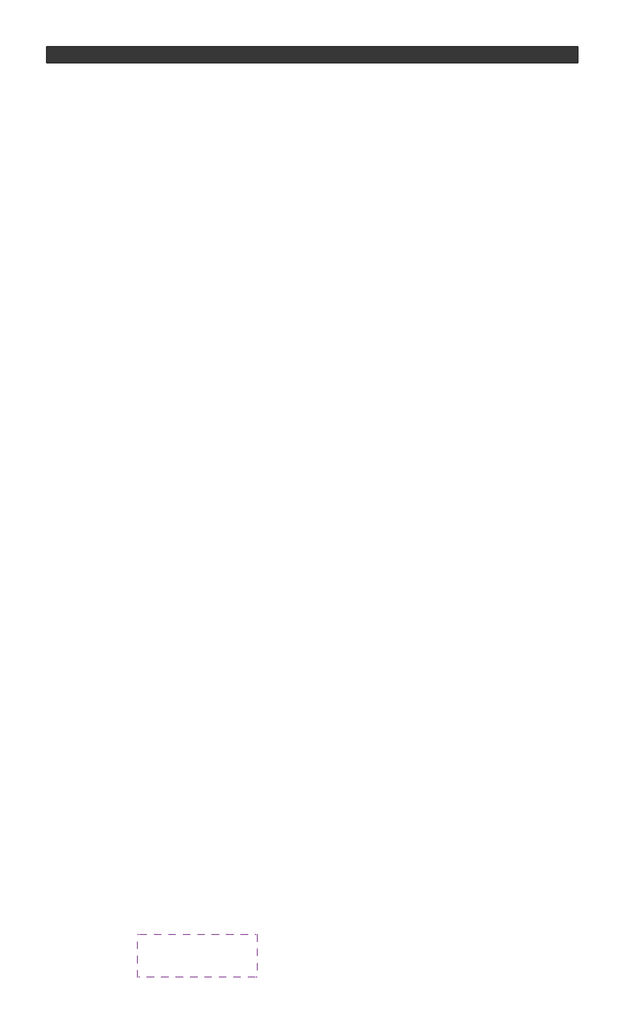
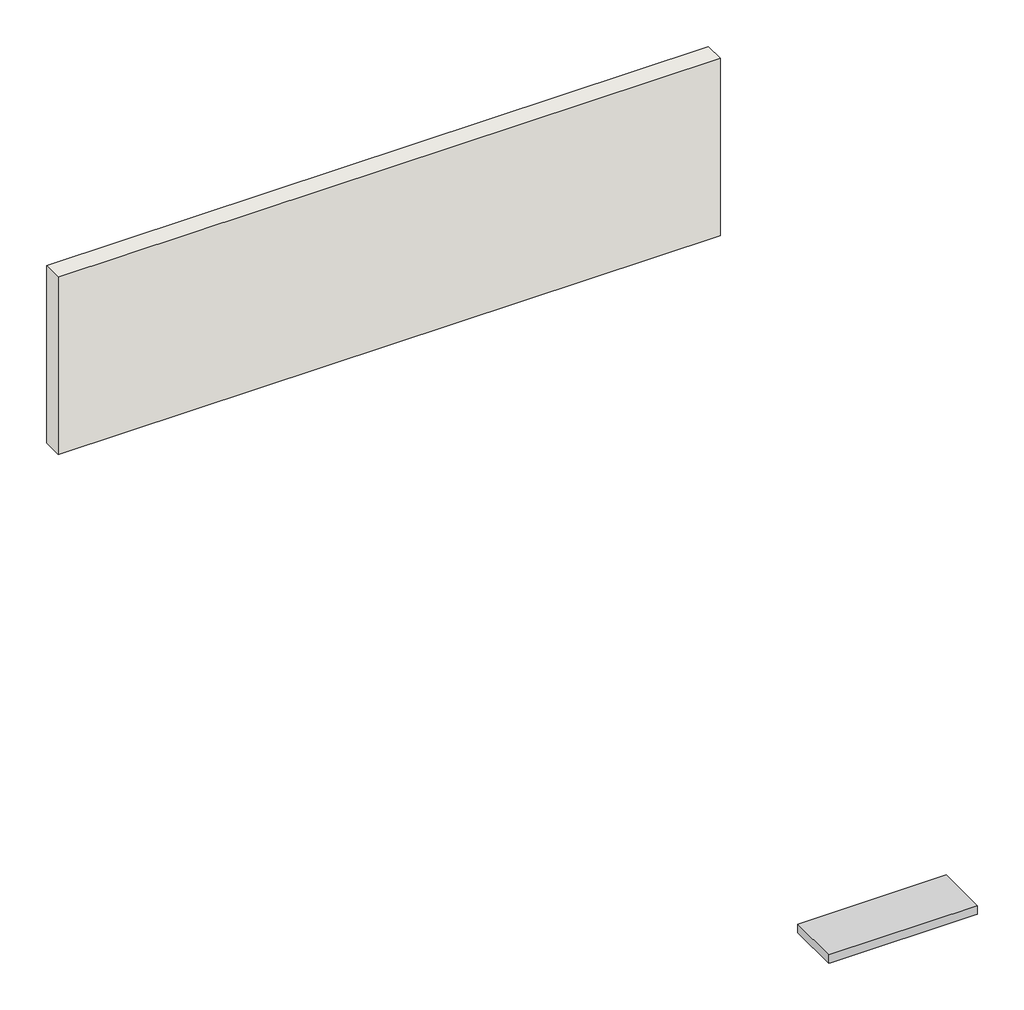
# One storey: 1 proxy, 1 wall.
"""IFC4 building model written with IfcOpenShell, lengths in millimetres."""

from ifc_helpers import new_model, si_unit, frame, origin, place, context, project, spatial, polyline, outline, extrude, transform, mapped, element, save
from components import generic_models_6_generic_models_6_bff87668

model = new_model("IFC4")

# Units and contexts
model_context = context("Model", 3, world=origin())
ifc_project = project(units=[si_unit("LENGTHUNIT", "METRE", prefix="MILLI")], contexts=[model_context])

# Site, building, storey
site = spatial("IfcSite", under=ifc_project)
building = spatial("IfcBuilding", under=site)
storey = spatial("IfcBuildingStorey", under=building, Elevation=3962.4)

# Proxy
placement = place(None, origin())
generic_models_6_generic_models_6_shape = generic_models_6_generic_models_6_bff87668(model_context)
element("IfcBuildingElementProxy", 1, Name="Generic Models 6 : Generic Models 6", ObjectType="Generic Models 6 : Generic Models 6", at=placement, inside=storey, context=model_context, shape_type="MappedRepresentation", body=[
    mapped(generic_models_6_generic_models_6_shape, transform((0.0, 0.0, 0.0), x_axis=(1.0, 0.0, 0.0), y_axis=(0.0, 1.0, 0.0), z_axis=(0.0, 0.0, 1.0))),
])

# Wall
element("IfcWall", 2, ObjectType="WALL 9\"", at=placement, inside=storey, context=model_context, shape_type="SweptSolid", body=[
    extrude(outline(polyline([(-735.1519453, 16291.0444012), (-8253.5519453, 16291.0444012), (-8253.5519453, 16519.6444012), (-735.1519453, 16519.6444012), (-735.1519453, 16291.0444012)])), frame((0.0, 0.0, 3962.4), z_axis=(0.0, 0.0, 1.0), x_axis=(1.0, 0.0, 0.0)), (0.0, 0.0, 1.0), 2133.6),
])

save(model, "model.ifc")

# Revit data of these elements
# Type "WALL 9\""
#   Assembly Code = "B2010"
#   Layers, outside or top first: 0' - 9" no material (function 1)
# Element 1 (IfcBuildingElementProxy, "Generic Models 6 : Generic Models 6")
#   Phase Created = New Construction
# Element 2 (IfcWall, "WALL 9\"")
#   Top Offset = 0' - 0"
#   Base Offset = 0' - 0"
#   wall height = 7' - 0"
#   Phase Created = New Construction
#   Top Constraint = FIRST FLOOR
#   Materials on its faces: "Default Wall", "1 wall paint"
# Materials
#   "Default Wall": colour RGB 128 128 128, transparency 0, Cost = 0
#   "1 wall paint": class "Generic", colour RGB 120 120 120, transparency 0, Cost = 0
